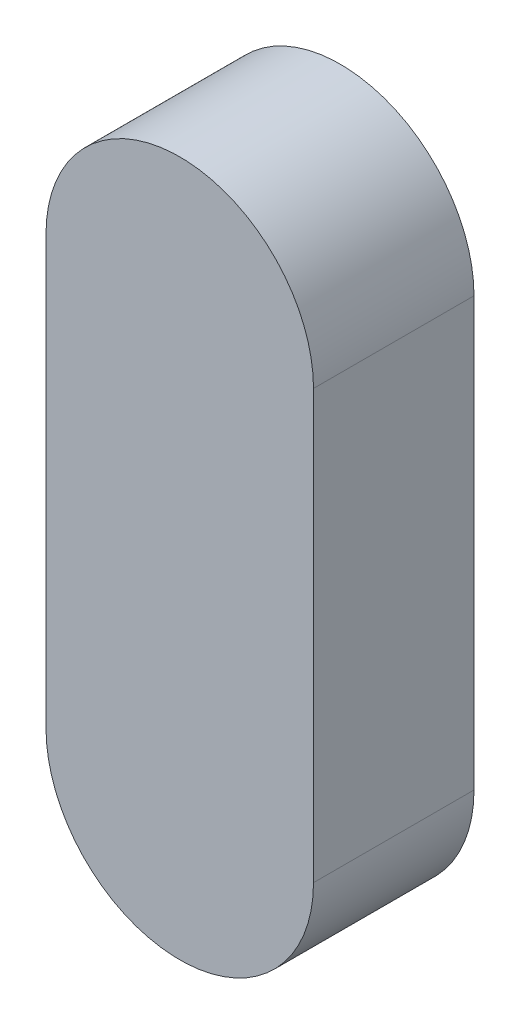
from build123d import *

# Parameters (mm, degrees)
KEY_BODY_3MM_DEPTH = 3


with BuildPart() as part:
    # Key Profile 5x13 → Key Body 3mm (new body)
    with BuildSketch(Plane.XY):
        with BuildLine():
            Line((-2.5, 0), (-2.5, 8))
            ThreePointArc((-2.5, 8), (0, 10.5), (2.5, 8))
            Line((2.5, 8), (2.5, 0))
            ThreePointArc((2.5, 0), (0, -2.5), (-2.5, 0))
        make_face()
    extrude(amount=KEY_BODY_3MM_DEPTH)


solid = part.part
